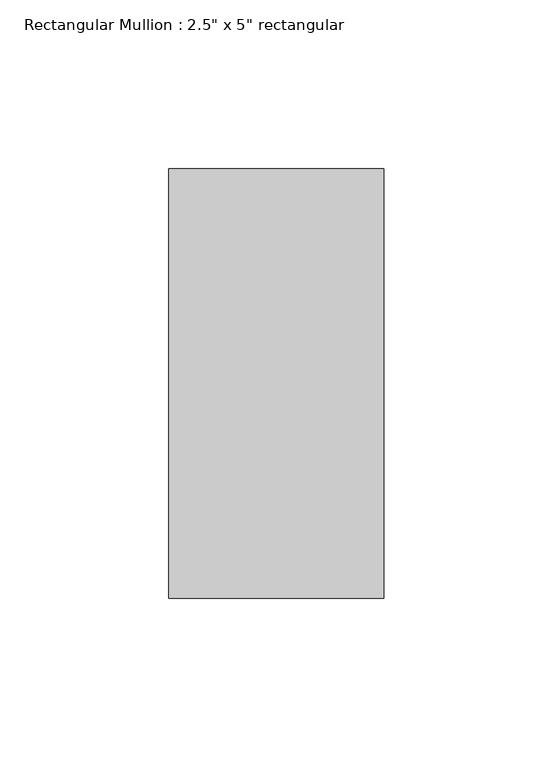
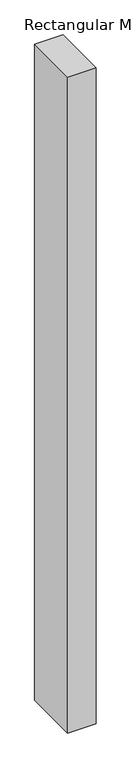
"""IFC4 building model written with IfcOpenShell, lengths in millimetres: member geometry."""

from ifc_helpers import new_model, si_unit, frame, origin, place, context, project, spatial, polyline, outline, extrude, source, transform, mapped, element, save


def member_31190633(model_context):
    return source(origin(), model_context, "Body", "SweptSolid", [
        extrude(outline(polyline([(31.75, 63.5), (31.75, -63.5), (-31.75, -63.5), (-31.75, 63.5), (31.75, 63.5)])), frame((0.0, 0.0, -1544.0388529), z_axis=(0.0, 0.0, 1.0), x_axis=(1.0, 0.0, 0.0)), (0.0, 0.0, 1.0), 1544.0388529),
    ])


if __name__ == "__main__":
    model = new_model("IFC4")
    model_context = context("Model", 3, world=origin())
    ifc_project = project(units=[si_unit("LENGTHUNIT", "METRE", prefix="MILLI")], contexts=[model_context])
    site = spatial("IfcSite", under=ifc_project)
    building = spatial("IfcBuilding", under=site)
    placement = place(None, origin())
    member_shape = member_31190633(model_context)
    element("IfcMember", 1, ObjectType="Rectangular Mullion : 2.5\" x 5\" rectangular", at=placement, inside=building, context=model_context, shape_type="MappedRepresentation", body=[
        mapped(member_shape, transform((0.0, 0.0, 0.0), x_axis=(1.0, 0.0, 0.0), y_axis=(0.0, 1.0, 0.0), z_axis=(0.0, 0.0, 1.0))),
    ])
    save(model, "model.ifc")

# Revit data of these elements
# Type "Rectangular Mullion : 2.5\" x 5\" rectangular"
#   built-in parameter 1007304 = 0.416667 (stored number, unit not read)
#   built-in parameter 1007301 = 0.104167 (stored number, unit not read)
#   built-in parameter 1007300 = 0.104167 (stored number, unit not read)
# Element 1 (IfcMember, "Rectangular Mullion : 2.5\" x 5\" rectangular")
#   Materials on its faces: "Aluminum"
# Materials
#   "Aluminum": class "Metal", colour RGB 247 247 247, transparency 0, Description = "Aluminum 6061", Cost = 0
